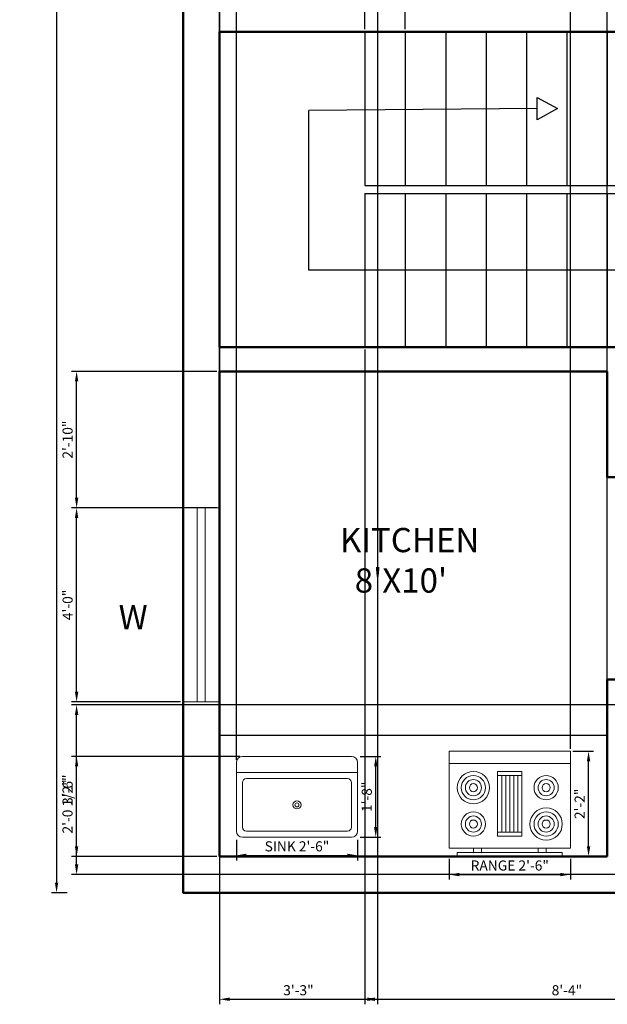
# Model space of a CAD drawing. Units: inches. Extents: x 2936 to 3364, y 2324 to 2867.
# Tile 1 of 4: x 2936 to 3081, y 2325 to 2568. Entities that reach past the tile are written whole.
import ezdxf

# ---------------------------------------------------------------- set-up
doc = ezdxf.new("R2010")
doc.units = ezdxf.units.IN
for name, color, linetype, lineweight in [('A-ANNO-DIMS', 2, 'Continuous', 18), ('A-ANNO-TEXT', 7, 'Continuous', 18), ('A-AREA-IDEN', 7, 'Continuous', 25), ('A-EQPM', 8, 'Continuous', 18), ('A-FLOR-CASE', 9, 'Continuous', 25), ('A-FLOR-FIXT', 9, 'Continuous', 18), ('A-FLOR-STRS', 7, 'Continuous', 25), ('A-GLAZ', 4, 'Continuous', 18), ('A-WALL', 7, 'Continuous', 50)]:
    doc.layers.add(name, color=color, linetype=linetype, lineweight=lineweight)
doc.styles.get("Standard").update_dxf_attribs({"font": 'arial.ttf'})
doc.dimstyles.new('ISO-25', dxfattribs={"dimtxt": 2.5, "dimasz": 2.5, "dimexe": 1.25, "dimexo": 0.625, "dimtad": 1, "dimdec": 0, "dimlunit": 4, "dimtxsty": 'Standard', "dimcen": 2.5, "dimadec": 0, "dimazin": 0, "dimtfac": 1, "dimtdec": 0, "dimtmove": 0, "dimatfit": 3, "dimfxl": 1, "dimarcsym": 0})

# ---------------------------------------------------------------- blocks, each defined once
blk = doc.blocks.new('Sink-single - 30 in top')
blk.add_line((-15, -3.999996), (15, -3.999996))
for points in [[(-13.5, 0), (13.5, 0)], [(-15, -18.499996), (-15, -1.5)], [(15, -1.5), (15, -18.499996)], [(-13.5, -17.499996), (-13.5, -6.499996)], [(-12.5, -5.499996), (12.5, -5.499996)], [(13.5, -6.499996), (13.5, -17.499996)], [(12.5, -18.499996), (-12.5, -18.499996)], [(13.5, -19.999996), (-13.5, -19.999996)]]:
    blk.add_lwpolyline(points)
for radius in [1, 0.5]:
    blk.add_circle((0, -11.999996), radius)
for centre, radius, start, end in [((-13.5, -1.5), 1.5, 90, 180), ((13.5, -1.5), 1.5, 0, 90), ((-12.5, -6.499996), 1, 90, 180), ((12.5, -6.499996), 1, 0, 90), ((-13.5, -18.499996), 1.5, 180, 270), ((-12.5, -17.499996), 1, 180, 270), ((12.5, -17.499996), 1, 270, 0), ((13.5, -18.499996), 1.5, 270, 0)]:
    blk.add_arc(centre, radius, start, end)
blk = doc.blocks.new('Range-Oven - 30 in top')
for p, q in [((0, -3), (30, -3)), ((12, -6), (18, -6)), ((13, -20), (13, -6)), ((14, -6), (14, -20)), ((15, -20), (15, -6)), ((16, -6), (16, -20)), ((17, -20), (17, -6)), ((18, -20), (12, -20)), ((6, -24), (6, -25)), ((8, -25), (8, -24)), ((22, -25), (22, -24)), ((24, -24), (24, -25))]:
    blk.add_line(p, q)
for points in [[(0, -24), (0, 0), (30, 0), (30, -24)], [(12, -21), (12, -5), (18, -5), (18, -21)], [(2, -26), (2, -25), (28, -25), (28, -26)]]:
    blk.add_lwpolyline(points, close=True)
for centre, radius in [((6, -9), 4), ((6, -9), 3), ((6, -9), 2), ((24, -9), 3), ((24, -9), 2), ((6, -9), 1), ((24, -9), 1), ((24, -18), 4), ((6, -18), 3), ((6, -18), 2), ((6, -18), 1), ((24, -18), 3), ((24, -18), 2), ((24, -18), 1)]:
    blk.add_circle(centre, radius)
blk = doc.blocks.new('*D10')
at = {"layer": 'A-ANNO-DIMS', "color": 0, "lineweight": -2, "transparency": 16777216}
for p, q in [((2947.52, 2832.11), (2943.61, 2832.11)), ((2944.86, 2829.61), (2944.86, 2354.61)), ((2947.52, 2352.11), (2943.61, 2352.11))]:
    blk.add_line(p, q, dxfattribs=at)
at = {"layer": 'A-ANNO-DIMS', "color": 0, "transparency": 16777216}
for points in [[(2944.44, 2829.61), (2945.27, 2829.61), (2944.86, 2832.11)], [(2944.44, 2354.61), (2945.27, 2354.61), (2944.86, 2352.11)]]:
    blk.add_solid(points, dxfattribs=at)
at = {"layer": 'Defpoints', "color": 0, "transparency": 16777216}
for p in [(2948.14, 2832.11), (2944.86, 2352.11), (2948.14, 2352.11)]:
    blk.add_point(p, dxfattribs=at)
at = {"layer": 'A-ANNO-DIMS', "color": 0, "transparency": 16777216, "insert": (2940.15, 2592.11), "char_height": 2.5, "width": 21.2299, "attachment_point": 5, "rotation": 90}
blk.add_mtext("{\\H3.2x;40'}", dxfattribs=at)
blk = doc.blocks.new('*D33')
at = {"layer": 'A-ANNO-DIMS', "color": 0, "lineweight": -2, "transparency": 16777216}
for p, q in [((2989.36, 2365.23), (2989.36, 2360.1)), ((3019.36, 2365.23), (3019.36, 2360.1)), ((2991.86, 2361.35), (3016.86, 2361.35))]:
    blk.add_line(p, q, dxfattribs=at)
at = {"layer": 'A-ANNO-DIMS', "color": 0, "transparency": 16777216}
for points in [[(2991.86, 2361.77), (2991.86, 2360.94), (2989.36, 2361.35)], [(3016.86, 2361.77), (3016.86, 2360.94), (3019.36, 2361.35)]]:
    blk.add_solid(points, dxfattribs=at)
at = {"layer": 'Defpoints', "color": 0, "transparency": 16777216}
for p in [(2989.36, 2365.85), (3019.36, 2365.85), (3019.36, 2361.35)]:
    blk.add_point(p, dxfattribs=at)
at = {"layer": 'A-ANNO-DIMS', "color": 0, "transparency": 16777216, "insert": (3004.36, 2363.27), "char_height": 2.5, "attachment_point": 5}
blk.add_mtext('SINK 2\'-6"', dxfattribs=at)
blk = doc.blocks.new('*D34')
at = {"layer": 'A-ANNO-DIMS', "color": 0, "lineweight": -2, "transparency": 16777216}
for p, q in [((3019.99, 2385.85), (3025.11, 2385.85)), ((3023.86, 2368.35), (3023.86, 2383.35)), ((3019.99, 2365.85), (3025.11, 2365.85))]:
    blk.add_line(p, q, dxfattribs=at)
at = {"layer": 'A-ANNO-DIMS', "color": 0, "transparency": 16777216}
for points in [[(3023.45, 2383.35), (3024.28, 2383.35), (3023.86, 2385.85)], [(3023.45, 2368.35), (3024.28, 2368.35), (3023.86, 2365.85)]]:
    blk.add_solid(points, dxfattribs=at)
at = {"layer": 'Defpoints', "color": 0, "transparency": 16777216}
for p in [(3019.36, 2385.85), (3023.86, 2385.85), (3019.36, 2365.85)]:
    blk.add_point(p, dxfattribs=at)
at = {"layer": 'A-ANNO-DIMS', "color": 0, "transparency": 16777216, "insert": (3021.96, 2375.85), "char_height": 2.5, "attachment_point": 5, "rotation": 90}
blk.add_mtext('1\'-8"', dxfattribs=at)
blk = doc.blocks.new('*D35')
at = {"layer": 'A-ANNO-DIMS', "color": 0, "lineweight": -2, "transparency": 16777216}
for p, q in [((3042.03, 2360.49), (3042.03, 2355.36)), ((3072.03, 2360.49), (3072.03, 2355.36)), ((3044.53, 2356.61), (3069.53, 2356.61))]:
    blk.add_line(p, q, dxfattribs=at)
at = {"layer": 'A-ANNO-DIMS', "color": 0, "transparency": 16777216}
for points in [[(3044.53, 2357.03), (3044.53, 2356.2), (3042.03, 2356.61)], [(3069.53, 2357.03), (3069.53, 2356.2), (3072.03, 2356.61)]]:
    blk.add_solid(points, dxfattribs=at)
at = {"layer": 'Defpoints', "color": 0, "transparency": 16777216}
for p in [(3042.03, 2361.11), (3072.03, 2361.11), (3072.03, 2356.61)]:
    blk.add_point(p, dxfattribs=at)
at = {"layer": 'A-ANNO-DIMS', "color": 0, "transparency": 16777216, "insert": (3057.03, 2358.53), "char_height": 2.5, "attachment_point": 5}
blk.add_mtext('RANGE 2\'-6"', dxfattribs=at)
blk = doc.blocks.new('*D36')
at = {"layer": 'A-ANNO-DIMS', "color": 0, "lineweight": -2, "transparency": 16777216}
for p, q in [((3072.66, 2387.11), (3077.78, 2387.11)), ((3076.53, 2363.61), (3076.53, 2384.61)), ((3072.66, 2361.11), (3077.78, 2361.11))]:
    blk.add_line(p, q, dxfattribs=at)
at = {"layer": 'A-ANNO-DIMS', "color": 0, "transparency": 16777216}
for points in [[(3076.11, 2384.61), (3076.95, 2384.61), (3076.53, 2387.11)], [(3076.11, 2363.61), (3076.95, 2363.61), (3076.53, 2361.11)]]:
    blk.add_solid(points, dxfattribs=at)
at = {"layer": 'Defpoints', "color": 0, "transparency": 16777216}
for p in [(3072.03, 2387.11), (3076.53, 2387.11), (3072.03, 2361.11)]:
    blk.add_point(p, dxfattribs=at)
at = {"layer": 'A-ANNO-DIMS', "color": 0, "transparency": 16777216, "insert": (3074.65, 2374.11), "char_height": 2.5, "attachment_point": 5, "rotation": 90}
blk.add_mtext('2\'-2"', dxfattribs=at)
blk = doc.blocks.new('*D38')
at = {"layer": 'A-ANNO-DIMS', "color": 0, "lineweight": -2, "transparency": 16777216}
for p, q in [((2975.54, 2447.33), (2948.57, 2447.33)), ((2949.82, 2401.83), (2949.82, 2444.83)), ((2975.54, 2399.33), (2948.57, 2399.33))]:
    blk.add_line(p, q, dxfattribs=at)
at = {"layer": 'A-ANNO-DIMS', "color": 0, "transparency": 16777216}
for points in [[(2949.4, 2444.83), (2950.24, 2444.83), (2949.82, 2447.33)], [(2949.4, 2401.83), (2950.24, 2401.83), (2949.82, 2399.33)]]:
    blk.add_solid(points, dxfattribs=at)
at = {"layer": 'Defpoints', "color": 0, "transparency": 16777216}
for p in [(2949.82, 2447.33), (2976.17, 2447.33), (2976.17, 2399.33)]:
    blk.add_point(p, dxfattribs=at)
at = {"layer": 'A-ANNO-DIMS', "color": 0, "transparency": 16777216, "insert": (2947.92, 2423.33), "char_height": 2.5, "attachment_point": 5, "rotation": 90}
blk.add_mtext('4\'-0"', dxfattribs=at)
blk = doc.blocks.new('*D39')
at = {"layer": 'A-ANNO-DIMS', "color": 0, "lineweight": -2, "transparency": 16777216}
for p, q in [((2984.54, 2481.11), (2948.57, 2481.11)), ((2949.82, 2449.83), (2949.82, 2478.61)), ((2984.54, 2447.33), (2948.57, 2447.33))]:
    blk.add_line(p, q, dxfattribs=at)
at = {"layer": 'A-ANNO-DIMS', "color": 0, "transparency": 16777216}
for points in [[(2949.4, 2478.61), (2950.24, 2478.61), (2949.82, 2481.11)], [(2949.4, 2449.83), (2950.24, 2449.83), (2949.82, 2447.33)]]:
    blk.add_solid(points, dxfattribs=at)
at = {"layer": 'Defpoints', "color": 0, "transparency": 16777216}
for p in [(2949.82, 2481.11), (2985.17, 2481.11), (2985.17, 2447.33)]:
    blk.add_point(p, dxfattribs=at)
at = {"layer": 'A-ANNO-DIMS', "color": 0, "transparency": 16777216, "insert": (2947.92, 2464.22), "char_height": 2.5, "attachment_point": 5, "rotation": 90}
blk.add_mtext('2\'-10"', dxfattribs=at)
blk = doc.blocks.new('*D43')
at = {"layer": 'A-ANNO-DIMS', "color": 0, "lineweight": -2, "transparency": 16777216}
for p, q in [((2985.17, 2822.49), (2985.17, 2324.51)), ((3024.27, 2822.49), (3024.27, 2324.51)), ((2987.67, 2325.76), (3021.77, 2325.76))]:
    blk.add_line(p, q, dxfattribs=at)
at = {"layer": 'A-ANNO-DIMS', "color": 0, "transparency": 16777216}
for points in [[(2987.67, 2326.18), (2987.67, 2325.35), (2985.17, 2325.76)], [(3021.77, 2326.18), (3021.77, 2325.35), (3024.27, 2325.76)]]:
    blk.add_solid(points, dxfattribs=at)
at = {"layer": 'Defpoints', "color": 0, "transparency": 16777216}
for p in [(2985.17, 2823.11), (3024.27, 2823.11), (3024.27, 2325.76)]:
    blk.add_point(p, dxfattribs=at)
at = {"layer": 'A-ANNO-DIMS', "color": 0, "transparency": 16777216, "insert": (3004.72, 2327.67), "char_height": 2.5, "attachment_point": 5}
blk.add_mtext('3\'-3"', dxfattribs=at)
blk = doc.blocks.new('*D48')
at = {"layer": 'A-ANNO-DIMS', "color": 0, "lineweight": -2, "transparency": 16777216}
for p, q in [((2985.17, 2565.74), (2985.17, 2859.71)), ((2987.67, 2858.46), (3018.67, 2858.46)), ((3021.17, 2565.74), (3021.17, 2859.71))]:
    blk.add_line(p, q, dxfattribs=at)
at = {"layer": 'A-ANNO-DIMS', "color": 0, "transparency": 16777216}
for points in [[(2987.67, 2858.88), (2987.67, 2858.05), (2985.17, 2858.46)], [(3018.67, 2858.88), (3018.67, 2858.05), (3021.17, 2858.46)]]:
    blk.add_solid(points, dxfattribs=at)
at = {"layer": 'Defpoints', "color": 0, "transparency": 16777216}
for p in [(3021.17, 2858.46), (2985.17, 2565.11), (3021.17, 2565.11)]:
    blk.add_point(p, dxfattribs=at)
at = {"layer": 'A-ANNO-DIMS', "color": 0, "transparency": 16777216, "insert": (3003.17, 2860.37), "char_height": 2.5, "attachment_point": 5}
blk.add_mtext('3\'-0"', dxfattribs=at)
blk = doc.blocks.new('*D49')
at = {"layer": 'A-ANNO-DIMS', "color": 0, "lineweight": -2, "transparency": 16777216}
for p, q in [((3021.17, 2565.74), (3021.17, 2859.71)), ((3023.67, 2858.46), (3028.67, 2858.46)), ((3031.17, 2565.74), (3031.17, 2859.71))]:
    blk.add_line(p, q, dxfattribs=at)
at = {"layer": 'A-ANNO-DIMS', "color": 0, "transparency": 16777216}
for points in [[(3023.67, 2858.88), (3023.67, 2858.05), (3021.17, 2858.46)], [(3028.67, 2858.88), (3028.67, 2858.05), (3031.17, 2858.46)]]:
    blk.add_solid(points, dxfattribs=at)
at = {"layer": 'Defpoints', "color": 0, "transparency": 16777216}
for p in [(3031.17, 2858.46), (3021.17, 2565.11), (3031.17, 2565.11)]:
    blk.add_point(p, dxfattribs=at)
at = {"layer": 'A-ANNO-DIMS', "color": 0, "transparency": 16777216, "insert": (3026.17, 2860.37), "char_height": 2.5, "attachment_point": 5}
blk.add_mtext('0\'-10"', dxfattribs=at)
blk = doc.blocks.new('*D58')
at = {"layer": 'A-ANNO-DIMS', "color": 0, "lineweight": -2, "transparency": 16777216}
for p, q in [((3021.17, 2486.49), (3021.17, 2324.51)), ((3121.17, 2486.49), (3121.17, 2324.51)), ((3023.67, 2325.76), (3118.67, 2325.76))]:
    blk.add_line(p, q, dxfattribs=at)
at = {"layer": 'A-ANNO-DIMS', "color": 0, "transparency": 16777216}
for points in [[(3023.67, 2326.18), (3023.67, 2325.35), (3021.17, 2325.76)], [(3118.67, 2326.18), (3118.67, 2325.35), (3121.17, 2325.76)]]:
    blk.add_solid(points, dxfattribs=at)
at = {"layer": 'Defpoints', "color": 0, "transparency": 16777216}
for p in [(3021.17, 2487.11), (3121.17, 2487.11), (3121.17, 2325.76)]:
    blk.add_point(p, dxfattribs=at)
at = {"layer": 'A-ANNO-DIMS', "color": 0, "transparency": 16777216, "insert": (3071.17, 2327.67), "char_height": 2.5, "attachment_point": 5}
blk.add_mtext('8\'-4"', dxfattribs=at)
blk = doc.blocks.new('*D61')
at = {"layer": 'A-ANNO-DIMS', "color": 0, "lineweight": -2, "transparency": 16777216}
for p, q in [((2982.67, 2858.46), (2980.17, 2858.46)), ((2985.17, 2391.74), (2985.17, 2859.71)), ((2985.17, 2858.46), (2989.36, 2858.46)), ((2989.36, 2384.98), (2989.36, 2859.71)), ((2991.86, 2858.46), (3002.26, 2858.46))]:
    blk.add_line(p, q, dxfattribs=at)
at = {"layer": 'A-ANNO-DIMS', "color": 0, "transparency": 16777216}
for points in [[(2982.67, 2858.88), (2982.67, 2858.05), (2985.17, 2858.46)], [(2991.86, 2858.88), (2991.86, 2858.05), (2989.36, 2858.46)]]:
    blk.add_solid(points, dxfattribs=at)
at = {"layer": 'Defpoints', "color": 0, "transparency": 16777216}
for p in [(2989.36, 2858.46), (2985.17, 2391.11), (2989.36, 2384.35)]:
    blk.add_point(p, dxfattribs=at)
at = {"layer": 'A-ANNO-DIMS', "color": 0, "transparency": 16777216, "insert": (2998.31, 2860.37), "char_height": 2.5, "attachment_point": 5}
blk.add_mtext('0\'-4"', dxfattribs=at)
blk = doc.blocks.new('*D62')
at = {"layer": 'A-ANNO-DIMS', "color": 0, "lineweight": -2, "transparency": 16777216}
for p, q in [((3072.03, 2387.74), (3072.03, 2859.71)), ((3078.67, 2858.46), (3074.53, 2858.46)), ((3081.17, 2391.74), (3081.17, 2859.71))]:
    blk.add_line(p, q, dxfattribs=at)
at = {"layer": 'A-ANNO-DIMS', "color": 0, "transparency": 16777216}
for points in [[(3074.53, 2858.88), (3074.53, 2858.05), (3072.03, 2858.46)], [(3078.67, 2858.88), (3078.67, 2858.05), (3081.17, 2858.46)]]:
    blk.add_solid(points, dxfattribs=at)
at = {"layer": 'Defpoints', "color": 0, "transparency": 16777216}
for p in [(3072.03, 2858.46), (3081.17, 2391.11), (3072.03, 2387.11)]:
    blk.add_point(p, dxfattribs=at)
at = {"layer": 'A-ANNO-DIMS', "color": 0, "transparency": 16777216, "insert": (3076.6, 2860.37), "char_height": 2.5, "attachment_point": 5}
blk.add_mtext('0\'-9"', dxfattribs=at)
blk = doc.blocks.new('*D63')
at = {"layer": 'A-ANNO-DIMS', "color": 0, "lineweight": -2, "transparency": 16777216}
for p, q in [((2990.24, 2385.85), (2948.57, 2385.85)), ((2949.82, 2363.61), (2949.82, 2383.35)), ((2984.54, 2361.11), (2948.57, 2361.11))]:
    blk.add_line(p, q, dxfattribs=at)
at = {"layer": 'A-ANNO-DIMS', "color": 0, "transparency": 16777216}
for points in [[(2949.4, 2383.35), (2950.24, 2383.35), (2949.82, 2385.85)], [(2949.4, 2363.61), (2950.24, 2363.61), (2949.82, 2361.11)]]:
    blk.add_solid(points, dxfattribs=at)
at = {"layer": 'Defpoints', "color": 0, "transparency": 16777216}
for p in [(2949.82, 2385.85), (2990.86, 2385.85), (2985.17, 2361.11)]:
    blk.add_point(p, dxfattribs=at)
at = {"layer": 'A-ANNO-DIMS', "color": 0, "transparency": 16777216, "insert": (2947.9, 2373.48), "char_height": 2.5, "attachment_point": 5, "rotation": 90}
blk.add_mtext('2\'-0 1/2"', dxfattribs=at)
blk = doc.blocks.new('*D64')
at = {"layer": 'A-ANNO-DIMS', "color": 0, "lineweight": -2, "transparency": 16777216}
for p, q in [((3324.54, 2398.61), (2948.57, 2398.61)), ((2949.82, 2359.11), (2949.82, 2396.11)), ((3324.54, 2356.61), (2948.57, 2356.61))]:
    blk.add_line(p, q, dxfattribs=at)
at = {"layer": 'A-ANNO-DIMS', "color": 0, "transparency": 16777216}
for points in [[(2949.4, 2396.11), (2950.24, 2396.11), (2949.82, 2398.61)], [(2949.4, 2359.11), (2950.24, 2359.11), (2949.82, 2356.61)]]:
    blk.add_solid(points, dxfattribs=at)
at = {"layer": 'Defpoints', "color": 0, "transparency": 16777216}
for p in [(2949.82, 2398.61), (3325.17, 2398.61), (3325.17, 2356.61)]:
    blk.add_point(p, dxfattribs=at)
at = {"layer": 'A-ANNO-DIMS', "color": 0, "transparency": 16777216, "insert": (2947.92, 2377.61), "char_height": 2.5, "attachment_point": 5, "rotation": 90}
blk.add_mtext('3\'-6"', dxfattribs=at)

msp = doc.modelspace()

# ---------------------------------------------------------------- linework, layer by layer
at = {"layer": 'A-FLOR-CASE'}
msp.add_line((2985.17, 2391.11), (3081.17, 2391.11), dxfattribs=at)
at = {"layer": 'A-FLOR-STRS'}
for p, q in [((3021.17, 2565.11), (3021.17, 2527.11)), ((3031.17, 2565.11), (3031.17, 2527.11)), ((3041.17, 2565.11), (3041.17, 2527.11)), ((3051.17, 2565.11), (3051.17, 2527.11)), ((3061.17, 2565.11), (3061.17, 2527.11)), ((3071.17, 2565.11), (3071.17, 2527.11)), ((3081.17, 2565.11), (3081.17, 2527.11)), ((3063.83, 2548.87), (3068.88, 2546.11)), ((3063.85, 2546.11), (3007.29, 2545.61)), ((3068.88, 2546.11), (3063.83, 2543.35)), ((3007.29, 2506.11), (3007.29, 2545.61)), ((3021.17, 2527.11), (3121.17, 2527.11)), ((3021.17, 2525.11), (3121.17, 2525.11)), ((3021.17, 2525.11), (3021.17, 2487.11)), ((3031.17, 2525.11), (3031.17, 2487.11)), ((3041.17, 2525.11), (3041.17, 2487.11)), ((3051.17, 2525.11), (3051.17, 2487.11)), ((3061.17, 2525.11), (3061.17, 2487.11)), ((3071.17, 2525.11), (3071.17, 2487.11)), ((3081.17, 2525.11), (3081.17, 2487.11)), ((3091.17, 2506.11), (3007.29, 2506.11))]:
    msp.add_line(p, q, dxfattribs=at)
msp.add_lwpolyline([(3063.83, 2543.35), (3063.83, 2548.87)], dxfattribs=at)
at = {"layer": 'A-GLAZ'}
for p, q in [((2985.17, 2447.33), (2976.17, 2447.33)), ((2979.67, 2447.33), (2979.67, 2399.33)), ((2981.67, 2447.33), (2981.67, 2399.33)), ((2985.17, 2399.33), (2976.17, 2399.33))]:
    msp.add_line(p, q, dxfattribs=at)
at = {"layer": 'A-WALL'}
for p, q in [((3111.17, 2565.11), (2985.17, 2565.11)), ((2985.17, 2565.11), (2985.17, 2487.11)), ((2985.17, 2487.11), (3121.17, 2487.11)), ((2985.17, 2481.11), (3081.17, 2481.11)), ((2985.17, 2481.11), (2985.17, 2361.11)), ((3081.17, 2481.11), (3081.17, 2454.95)), ((3081.17, 2454.95), (3087.17, 2454.95)), ((3081.17, 2404.87), (3087.17, 2404.87)), ((3081.17, 2404.87), (3081.17, 2361.11)), ((2985.17, 2361.11), (3081.17, 2361.11))]:
    msp.add_line(p, q, dxfattribs=at)
msp.add_lwpolyline([(3336.17, 2352.11), (3336.17, 2832.11), (2976.17, 2832.11), (2976.17, 2352.11), (3279.17, 2352.11)], dxfattribs=at)

# ---------------------------------------------------------------- block references
at = {"layer": 'A-EQPM'}
msp.add_blockref('Range-Oven - 30 in top', (3042.03, 2387.11), dxfattribs=at)
at = {"layer": 'A-FLOR-FIXT'}
msp.add_blockref('Sink-single - 30 in top', (3004.36, 2385.85), dxfattribs=at)

# ---------------------------------------------------------------- texts
at = {"layer": 'A-ANNO-TEXT', "insert": (2960.22, 2423.3), "char_height": 6, "attachment_point": 1}
msp.add_mtext_dynamic_manual_height_columns('W', width=56.3393, gutter_width=12.5, heights=[0], dxfattribs=at)
at = {"layer": 'A-AREA-IDEN', "insert": (3014.99, 2442.37), "char_height": 6, "attachment_point": 1}
msp.add_mtext_dynamic_manual_height_columns("KITCHEN\\P  8'X10'", width=56.3393, gutter_width=12.5, heights=[0], dxfattribs=at)

# ---------------------------------------------------------------- dimensions: what is measured, and where the dimension line sits
at = {"layer": 'A-ANNO-DIMS'}
for base, p1, p2, picture, middle in [((2989.36, 2858.46), (2985.17, 2391.11), (2989.36, 2384.35), '*D61', (2998.31, 2860.37)), ((3021.17, 2858.46), (2985.17, 2565.11), (3021.17, 2565.11), '*D48', (3003.17, 2860.37)), ((3031.17, 2858.46), (3021.17, 2565.11), (3031.17, 2565.11), '*D49', (3026.17, 2860.37)), ((3072.03, 2858.46), (3081.17, 2391.11), (3072.03, 2387.11), '*D62', (3076.6, 2860.37)), ((3024.27, 2325.76), (2985.17, 2823.11), (3024.27, 2823.11), '*D43', (3004.72, 2327.67)), ((3121.17, 2325.76), (3021.17, 2487.11), (3121.17, 2487.11), '*D58', (3071.17, 2327.67))]:
    dim = msp.add_linear_dim(base=base, p1=p1, p2=p2, dimstyle='ISO-25', override={"dimdec": 1, "dimlfac": 1, "dimrnd": 0, "dimzin": 1, "dimdsep": 46, "dimlunit": 4, "dimfrac": 2}, dxfattribs=at)
    dim.commit()
    dim.dimension.update_dxf_attribs({"geometry": picture, "text_midpoint": middle})
dim = msp.add_linear_dim(base=(2944.86, 2352.11), p1=(2948.14, 2832.11), p2=(2948.14, 2352.11), angle=90, text='{\\H3.2x;<>}', dimstyle='ISO-25', override={"dimclrd": 0, "dimclre": 0, "dimclrt": 0}, dxfattribs=at)
dim.commit()
dim.dimension.update_dxf_attribs({"geometry": '*D10', "text_midpoint": (2940.15, 2592.11)})
for base, p1, p2, picture, middle in [((2949.82, 2481.11), (2985.17, 2447.33), (2985.17, 2481.11), '*D39', (2947.92, 2464.22)), ((2949.82, 2447.33), (2976.17, 2399.33), (2976.17, 2447.33), '*D38', (2947.92, 2423.33)), ((2949.82, 2398.61), (3325.17, 2356.61), (3325.17, 2398.61), '*D64', (2947.92, 2377.61)), ((2949.82, 2385.85), (2985.17, 2361.11), (2990.86, 2385.85), '*D63', (2947.9, 2373.48)), ((3023.86, 2385.85), (3019.36, 2365.85), (3019.36, 2385.85), '*D34', (3021.96, 2375.85)), ((3076.53, 2387.11), (3072.03, 2361.11), (3072.03, 2387.11), '*D36', (3074.65, 2374.11))]:
    dim = msp.add_linear_dim(base=base, p1=p1, p2=p2, angle=90, dimstyle='ISO-25', override={"dimdec": 1, "dimlfac": 1, "dimrnd": 0, "dimzin": 1, "dimdsep": 46, "dimlunit": 4, "dimfrac": 2}, dxfattribs=at)
    dim.commit()
    dim.dimension.update_dxf_attribs({"geometry": picture, "text_midpoint": middle})
for base, p1, p2, text, picture, middle in [((3019.36, 2361.35), (2989.36, 2365.85), (3019.36, 2365.85), 'SINK <>', '*D33', (3004.36, 2363.27)), ((3072.03, 2356.61), (3042.03, 2361.11), (3072.03, 2361.11), 'RANGE <>', '*D35', (3057.03, 2358.53))]:
    dim = msp.add_linear_dim(base=base, p1=p1, p2=p2, text=text, dimstyle='ISO-25', override={"dimdec": 1, "dimlfac": 1, "dimrnd": 0, "dimzin": 1, "dimdsep": 46, "dimlunit": 4, "dimfrac": 2}, dxfattribs=at)
    dim.commit()
    dim.dimension.update_dxf_attribs({"geometry": picture, "text_midpoint": middle})

doc.saveas('drawing.dxf')
